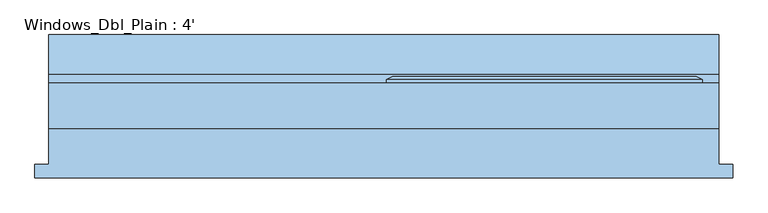
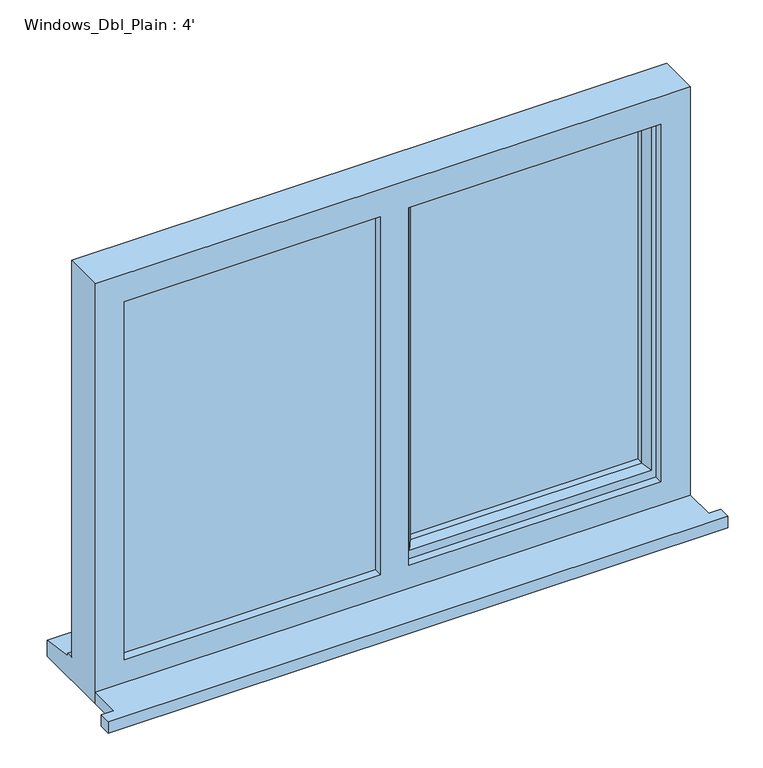
"""IFC4 building model written with IfcOpenShell, lengths in millimetres: window geometry, Windows_Dbl_Plain : 4'."""

from ifc_helpers import new_model, si_unit, frame, origin, place, context, project, spatial, polyline, outline, extrude, faceted_brep, source, transform, mapped, element, save


def windows_dbl_plain_4_e08ba9e4(model_context):
    return source(origin(), model_context, "Body", "SolidModel", [
        extrude(outline(polyline([(-919.6, -115.6034322), (-919.6, -90.6034322), (-894.6, -90.6034322), (-894.6, -25.4834322), (324.6, -25.4834322), (324.6, -90.6034322), (349.6, -90.6034322), (349.6, -115.6034322), (-919.6, -115.6034322)])), frame((0.0, 0.0, 1200.0), z_axis=(0.0, 0.0, 1.0), x_axis=(1.0, 0.0, 0.0)), (0.0, 0.0, 1.0), 25.0),
        faceted_brep([(-280.0, 57.5165678, 2080.0), (-280.0, 63.2900705, 2080.0), (-280.0, 63.2900705, 1253.0), (-280.0, 57.5165678, 1253.0), (-270.0, -7.4834322, 2070.0), (-270.0, 57.5165678, 2070.0), (-270.0, 57.5165678, 1263.0), (-270.0, -7.4834322, 1263.0), (-230.0, 7.0094677, 2030.0), (-240.1480377, -7.4834322, 2040.1480377), (-240.1480377, -7.4834322, 1292.8519623), (-230.0, 7.0094677, 1303.0), (-230.0, 21.5165678, 2030.0), (-230.0, 21.5165678, 1303.0), (-240.0, 45.5165678, 2040.0), (-240.0, 21.5165678, 2040.0), (-240.0, 21.5165678, 1293.0), (-240.0, 45.5165678, 1293.0), (-230.0, 63.2900705, 2030.0), (-230.0, 45.5165678, 2030.0), (-230.0, 45.5165678, 1303.0), (-230.0, 63.2900705, 1303.0), (-247.4457548, 69.0635732, 2047.4457548), (-247.4457548, 69.0635732, 1285.5542452), (-269.2153903, 69.0635732, 2069.2153903), (-269.2153903, 69.0635732, 1263.7846097), (294.6, 63.2900705, 1253.0), (294.6, 57.5165678, 1253.0), (284.6, 57.5165678, 1263.0), (284.6, -7.4834322, 1263.0), (254.7480377, -7.4834322, 1292.8519623), (244.6, 7.0094677, 1303.0), (244.6, 21.5165678, 1303.0), (254.6, 21.5165678, 1293.0), (254.6, 45.5165678, 1293.0), (244.6, 45.5165678, 1303.0), (244.6, 63.2900705, 1303.0), (262.0457548, 69.0635732, 1285.5542452), (283.8153903, 69.0635732, 1263.7846097), (294.6, 63.2900705, 2080.0), (294.6, 57.5165678, 2080.0), (284.6, 57.5165678, 2070.0), (284.6, -7.4834322, 2070.0), (254.7480377, -7.4834322, 2040.1480377), (244.6, 7.0094677, 2030.0), (244.6, 21.5165678, 2030.0), (254.6, 21.5165678, 2040.0), (254.6, 45.5165678, 2040.0), (244.6, 45.5165678, 2030.0), (244.6, 63.2900705, 2030.0), (262.0457548, 69.0635732, 2047.4457548), (283.8153903, 69.0635732, 2069.2153903)], [[[0, 1, 2, 3]], [[4, 5, 6, 7]], [[8, 9, 10, 11]], [[12, 8, 11, 13]], [[14, 15, 16, 17]], [[18, 19, 20, 21]], [[22, 18, 21, 23]], [[1, 24, 25, 2]], [[3, 2, 26, 27]], [[7, 6, 28, 29]], [[11, 10, 30, 31]], [[13, 11, 31, 32]], [[17, 16, 33, 34]], [[21, 20, 35, 36]], [[23, 21, 36, 37]], [[2, 25, 38, 26]], [[27, 26, 39, 40]], [[29, 28, 41, 42]], [[31, 30, 43, 44]], [[32, 31, 44, 45]], [[34, 33, 46, 47]], [[36, 35, 48, 49]], [[37, 36, 49, 50]], [[26, 38, 51, 39]], [[40, 39, 1, 0]], [[3, 27, 40, 0], [5, 41, 28, 6]], [[42, 41, 5, 4]], [[7, 29, 42, 4], [9, 43, 30, 10]], [[44, 43, 9, 8]], [[45, 44, 8, 12]], [[15, 46, 33, 16], [13, 32, 45, 12]], [[47, 46, 15, 14]], [[17, 34, 47, 14], [19, 48, 35, 20]], [[49, 48, 19, 18]], [[50, 49, 18, 22]], [[24, 51, 38, 25], [23, 37, 50, 22]], [[39, 51, 24, 1]]]),
        extrude(outline(polyline([(2050.0, -310.0), (2070.0, -310.0), (2070.0, -854.6), (1263.0, -854.6), (1263.0, -310.0), (1283.0, -310.0), (1283.0, -834.6), (2050.0, -834.6), (2050.0, -310.0)])), frame((0.0, 16.5165678, 0.0), z_axis=(0.0, 1.0, 0.0), x_axis=(0.0, 0.0, 1.0)), (0.0, 0.0, 1.0), 41.0),
        faceted_brep([(324.6, -25.4834322, 2110.0), (-894.6, -25.4834322, 2110.0), (-894.6, -25.4834322, 1200.0), (324.6, -25.4834322, 1200.0), (264.6, -25.4834322, 2050.0), (264.6, -25.4834322, 1275.0), (-252.0, -25.4834322, 1275.0), (-252.0, -25.4834322, 2050.0), (-310.0, -25.4834322, 2050.0), (-310.0, -25.4834322, 1275.0), (-834.6, -25.4834322, 1275.0), (-834.6, -25.4834322, 2050.0), (-894.6, 57.5165678, 2110.0), (-894.6, 57.5165678, 1251.0), (-894.6, 72.5165678, 1249.68767), (-894.6, 72.5165678, 1244.7449676), (-894.6, 145.0165678, 1233.8088847), (-894.6, 145.0165678, 1200.0), (324.6, 57.5165678, 2110.0), (324.6, 57.5165678, 1251.0), (-854.6, 57.5165678, 2070.0), (-854.6, 57.5165678, 1263.0), (-310.0, 57.5165678, 1263.0), (-310.0, 57.5165678, 2070.0), (-270.0, 57.5165678, 2070.0), (-270.0, 57.5165678, 1263.0), (284.6, 57.5165678, 1263.0), (284.6, 57.5165678, 2070.0), (-854.6, -7.4834322, 2070.0), (-854.6, -7.4834322, 1263.0), (-300.0, -7.4834322, 2070.0), (-300.0, -7.4834322, 1263.0), (-310.0, -7.4834322, 2050.0), (-834.6, -7.4834322, 2050.0), (-834.6, -7.4834322, 1275.0), (-310.0, -7.4834322, 1275.0), (-270.0, -7.4834322, 2070.0), (284.6, -7.4834322, 2070.0), (284.6, -7.4834322, 1263.0), (-270.0, -7.4834322, 1263.0), (264.6, -7.4834322, 2050.0), (-252.0, -7.4834322, 2050.0), (-252.0, -7.4834322, 1275.0), (264.6, -7.4834322, 1275.0), (-310.0, 16.5165678, 2070.0), (-300.0, 16.5165678, 2070.0), (324.6, 145.0165678, 1200.0), (324.6, 145.0165678, 1233.8088847), (324.6, 72.5165678, 1244.7449676), (324.6, 72.5165678, 1249.68767), (-300.0, 16.5165678, 1263.0), (-310.0, 16.5165678, 1263.0)], [[[0, 1, 2, 3], [4, 5, 6, 7], [8, 9, 10, 11]], [[2, 1, 12, 13, 14, 15, 16, 17]], [[13, 12, 18, 19], [20, 21, 22, 23], [24, 25, 26, 27]], [[21, 20, 28, 29]], [[28, 30, 31, 29], [32, 33, 34, 35]], [[36, 37, 38, 39], [40, 41, 42, 43]], [[33, 11, 10, 34]], [[1, 0, 18, 12]], [[28, 20, 23, 44, 45, 30]], [[27, 37, 36, 24]], [[11, 33, 32, 8]], [[40, 4, 7, 41]], [[19, 18, 0, 3, 46, 47, 48, 49]], [[27, 26, 38, 37]], [[4, 40, 43, 5]], [[45, 50, 31, 30]], [[50, 45, 44, 51]], [[51, 44, 23, 22]], [[25, 24, 36, 39]], [[41, 7, 6, 42]], [[8, 32, 35, 9]], [[46, 3, 2, 17]], [[47, 46, 17, 16]], [[48, 47, 16, 15]], [[49, 48, 15, 14]], [[19, 49, 14, 13]], [[22, 21, 29, 31, 50, 51]], [[26, 25, 39, 38]], [[6, 5, 43, 42]], [[35, 34, 10, 9]]]),
        extrude(outline(polyline([(-854.6, 16.5165678), (-300.0, 16.5165678), (-300.0, -7.4834322), (-854.6, -7.4834322), (-854.6, 16.5165678)])), frame((0.0, 0.0, 1263.0), z_axis=(0.0, 0.0, 1.0), x_axis=(1.0, 0.0, 0.0)), (0.0, 0.0, 1.0), 807.0),
        extrude(outline(polyline([(254.6, 21.5165678), (-240.0, 21.5165678), (-240.0, 45.5165678), (254.6, 45.5165678), (254.6, 21.5165678)])), frame((0.0, 0.0, 1293.0), z_axis=(0.0, 0.0, 1.0), x_axis=(1.0, 0.0, 0.0)), (0.0, 0.0, 1.0), 747.0),
    ])


if __name__ == "__main__":
    model = new_model("IFC4")
    model_context = context("Model", 3, world=origin())
    ifc_project = project(units=[si_unit("LENGTHUNIT", "METRE", prefix="MILLI")], contexts=[model_context])
    site = spatial("IfcSite", under=ifc_project)
    building = spatial("IfcBuilding", under=site)
    placement = place(None, origin())
    windows_dbl_plain_4_shape = windows_dbl_plain_4_e08ba9e4(model_context)
    element("IfcWindow", 1, ObjectType="Windows_Dbl_Plain : 4'", at=placement, inside=building, context=model_context, shape_type="MappedRepresentation", body=[
        mapped(windows_dbl_plain_4_shape, transform((0.0, 0.0, 0.0), x_axis=(1.0, 0.0, 0.0), y_axis=(0.0, 1.0, 0.0), z_axis=(0.0, 0.0, 1.0))),
    ])
    save(model, "model.ifc")

# Revit data of these elements
# Type "Windows_Dbl_Plain : 4'"
#   Type Mark = "56"
#   Operation = "DoublePanelVertical"
#   Construction Type Id = "GSP4R"
#   Manufacturer = "Revit"
#   Keynote = "L10"
#   Analytic Construction = "1/8 in Pilkington single glazing"
#   Wrap Layers (Ext) from Ext = 0.336286 ft
#   Wrap Layers (Int) from Ext = 0.582349 ft
#   Window Board Projection = 0.082021 ft
#   Window Board Extension = 0.082021 ft
#   Visual Light Transmittance = 0.9
#   Solar Heat Gain Coefficient = 0.78
#   Rough Width = 4.0 ft
#   Rough Height = 2.985564 ft
#   Height = 2.985564 ft
#   Width = 4.0 ft
#   Heat Transfer Coefficient (U) = 3.6886 W/(m²·K)
#   Glazing Thickness = 0.07874 ft
#   FrameOffset - External = 0.164042 ft
#   Frame Depth = 0.213255 ft
#   Default Head Height = 6.922572 ft
#   Cill Depth = 0.287073 ft
#   Cavity Closer Width = 0.164042 ft
#   Cavity Closer Offset from Ext = 0.336286 ft
#   Cavity Closer Depth = 0.278871 ft
#   Vis - Cavity Closers = yes
#   Define Thermal Properties by = 1
#   Material Trim = Window Frame
#   Material Glass = Glass
#   Material Frame = Window Frame
#   Wall Closure = (empty or 0)
# Element 1 (IfcWindow, "Windows_Dbl_Plain : 4'")
#   Materials on its faces: "Window Frame", "Glass"
# Materials
#   "Window Frame": colour RGB 249 249 249, transparency 0, Keynote = "L10", Cost = 0
#   "Glass": class "Glass", colour RGB 0 128 192, transparency 0.9, Description = "Soda Lime Glass", Cost = 0
